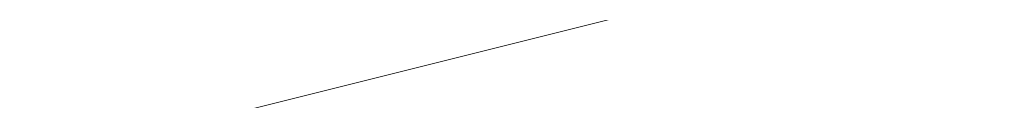
# Model space of a CAD drawing. Units: inches. Extents: x 2091 to 2899, y 967 to 2217.
# Tile 98 of 256: x 2251.243 to 2252.382, y 1099.986 to 1100.071. Entities that reach past the tile are written whole.
import ezdxf

# ---------------------------------------------------------------- set-up
doc = ezdxf.new("R2010")
doc.units = ezdxf.units.IN
doc.layers.add('A-ANNO-DIMS', color=2, linetype='Continuous', lineweight=18)
doc.layers.add('L-PLNT-TREE', color=94, linetype='Continuous', lineweight=13)
doc.layers.add('A-WALL-PATT', color=141, linetype='Continuous', lineweight=13, true_color=0xadddf7)
doc.styles.get("Standard").update_dxf_attribs({"font": 'arial.ttf'})
doc.dimstyles.new('ISO-25', dxfattribs={"dimtxt": 4, "dimasz": 4, "dimexe": 1.25, "dimexo": 0.625, "dimtad": 1, "dimdec": 0, "dimlunit": 3, "dimtxsty": 'Standard', "dimcen": 2.5, "dimadec": 0, "dimazin": 0, "dimtfac": 1, "dimtdec": 0, "dimtmove": 0, "dimatfit": 3, "dimfxl": 1, "dimarcsym": 0})

# ---------------------------------------------------------------- blocks, each defined once
blk = doc.blocks.new('*U29')
blk.add_line((-402.336, 12.192), (-451.104, 0))
blk = doc.blocks.new('*D71')
at = {"layer": 'A-ANNO-DIMS', "color": 0, "lineweight": -2, "transparency": 16777216}
for p, q in [((2212.1436, 1351.2941), (2212.1436, 969.4643)), ((2452.1436, 1351.2941), (2452.1436, 969.4643)), ((2216.1436, 970.7143), (2448.1436, 970.7143))]:
    blk.add_line(p, q, dxfattribs=at)
at = {"layer": 'A-ANNO-DIMS', "color": 0, "transparency": 16777216}
for points in [[(2216.1436, 971.381), (2216.1436, 970.0476), (2212.1436, 970.7143)], [(2448.1436, 971.381), (2448.1436, 970.0476), (2452.1436, 970.7143)]]:
    blk.add_solid(points, dxfattribs=at)
at = {"layer": 'Defpoints', "color": 0, "transparency": 16777216}
for p in [(2212.1436, 1351.9191), (2452.1436, 1351.9191), (2452.1436, 970.7143)]:
    blk.add_point(p, dxfattribs=at)
at = {"layer": 'A-ANNO-DIMS', "color": 0, "transparency": 16777216, "insert": (2332.1436, 973.3816), "char_height": 4, "attachment_point": 5}
blk.add_mtext('20\'-0"', dxfattribs=at)
blk = doc.blocks.new('*D75')
at = {"layer": 'A-ANNO-DIMS', "color": 0, "lineweight": -2, "transparency": 16777216}
for p, q in [((2212.1436, 1274.7941), (2212.1436, 969.4643)), ((2308.1436, 1274.7941), (2308.1436, 969.4643)), ((2216.1436, 970.7143), (2304.1436, 970.7143))]:
    blk.add_line(p, q, dxfattribs=at)
at = {"layer": 'A-ANNO-DIMS', "color": 0, "transparency": 16777216}
for points in [[(2216.1436, 971.381), (2216.1436, 970.0476), (2212.1436, 970.7143)], [(2304.1436, 971.381), (2304.1436, 970.0476), (2308.1436, 970.7143)]]:
    blk.add_solid(points, dxfattribs=at)
at = {"layer": 'Defpoints', "color": 0, "transparency": 16777216}
for p in [(2212.1436, 1275.4191), (2308.1436, 1275.4191), (2308.1436, 970.7143)]:
    blk.add_point(p, dxfattribs=at)
at = {"layer": 'A-ANNO-DIMS', "color": 0, "transparency": 16777216, "insert": (2260.1436, 973.3816), "char_height": 4, "attachment_point": 5}
blk.add_mtext('8\'-0"', dxfattribs=at)

msp = doc.modelspace()

# ---------------------------------------------------------------- hatches: boundary and pattern name
at = {"layer": 'A-WALL-PATT'}
h = msp.add_hatch(color=256, dxfattribs=at)
h.dxf.hatch_style = 1
h.paths.add_polyline_path([(2803.1436, 2050.9191), (2203.1436, 2050.9191), (2203.1436, 1090.9191), (2803.1436, 1090.9191)])
h.paths.add_polyline_path([(2635.7989, 1147.5405), (2674.5241, 1147.5405, 0.376086), (2678.5297, 1152.8802), (2678.5297, 1159.5565, 0.333335), (2674.5243, 1163.5618), (2674.5243, 1163.5619), (2674.5243, 1192.9344), (2635.806, 1192.9344), (2597.0876, 1192.9344), (2597.0876, 1163.5618, 0.333335), (2593.0823, 1159.5565), (2593.0823, 1152.8802, 0.376086), (2597.0879, 1147.5405)], flags=0)
h.paths.add_polyline_path([(2436.0104, 1278.2408, 0.000483), (2435.9526, 1278.215, -0.001328), (2435.9356, 1278.1117, -0.001711), (2436.1164, 1278.0408, 0.002185)], flags=0)
h.paths.add_polyline_path([(2794.1436, 1143.4191), (2794.1436, 1347.4191), (2543.3702, 1347.4191), (2543.3702, 1351.9191), (2794.1436, 1351.9191), (2794.1436, 1392.7136), (2793.9474, 1392.7136), (2793.9474, 1473.5369), (2794.1436, 1473.5369), (2794.1436, 1531.9191), (2650.1436, 1531.9191), (2650.1436, 1536.4191), (2794.1436, 1536.4191), (2794.1436, 1692.4191), (2609.3756, 1692.4191), (2609.3756, 1644.4191), (2604.8756, 1644.4191), (2604.8756, 1744.9191), (2609.3756, 1744.9191), (2609.3756, 1696.9191), (2794.1436, 1696.9191), (2794.1436, 1780.9191), (2609.6436, 1780.9191), (2493.8756, 1780.9191), (2493.8756, 1785.4191), (2609.6436, 1785.4191), (2794.1436, 1785.4191), (2794.1436, 1847.9388), (2793.9512, 1847.9388), (2793.9512, 1928.7622), (2794.1436, 1928.7622), (2794.1436, 1941.4191), (2614.1436, 1941.4191), (2614.1436, 1821.4191), (2609.6436, 1821.4191), (2609.6436, 1941.4191), (2392.1436, 1941.4191), (2392.1436, 1819.9191), (2387.6436, 1819.9191), (2387.6436, 1941.4191), (2212.1436, 1941.4191), (2212.1436, 1783.9191), (2392.1436, 1783.9191), (2392.1436, 1780.9191), (2212.1436, 1780.9191), (2212.1436, 1629.4191), (2387.6436, 1629.4191), (2387.6436, 1744.9191), (2392.1436, 1744.9191), (2392.1436, 1627.9191), (2317.1436, 1627.9191), (2317.1436, 1551.4191), (2317.1436, 1536.4191), (2459.3836, 1536.4191), (2459.3836, 1602.3965), (2463.8836, 1602.3965), (2463.8836, 1531.9191), (2456.6436, 1531.9191), (2456.6436, 1529.9191), (2452.1436, 1529.9191), (2452.1436, 1531.9191), (2312.6436, 1531.9191), (2312.6436, 1551.4191), (2306.1436, 1551.4191), (2306.1436, 1555.9191), (2308.1436, 1555.9191), (2308.1436, 1551.4191), (2312.6436, 1551.4191), (2312.6436, 1627.9191), (2212.1436, 1627.9191), (2212.1436, 1555.9191), (2270.1436, 1555.9191), (2270.1436, 1551.4191), (2212.1436, 1551.4191), (2212.1436, 1351.9191), (2272.1436, 1351.9191), (2272.1436, 1347.4191), (2212.1436, 1347.4191), (2212.1436, 1275.4191), (2308.1436, 1275.4191), (2308.1436, 1351.9191), (2452.1436, 1351.9191), (2452.1436, 1493.9191), (2456.6436, 1493.9191), (2456.6436, 1347.4191), (2312.6436, 1347.4191), (2312.6436, 1270.9191), (2212.1436, 1270.9191), (2212.1436, 1099.9191), (2281.2375, 1099.9191), (2282.871, 1110.9138), (2282.0083, 1116.9966), (2278.5577, 1121.4204), (2268.2056, 1128.0562), (2272.0876, 1128.0562), (2273.8129, 1131.927), (2279.4203, 1134.6919), (2285.0278, 1135.2449), (2287.6158, 1137.4568), (2288.0471, 1138.0098), (2289.3411, 1140.7747), (2291.0665, 1139.6687), (2292.3605, 1135.2449), (2295.3798, 1136.9038), (2296.2425, 1135.7979), (2297.1052, 1133.033), (2300.1246, 1138.0098), (2303.1439, 1138.0098), (2304.4379, 1135.7979), (2303.1439, 1133.586), (2306.5946, 1134.6919), (2307.8887, 1133.033), (2310.908, 1135.2449), (2313.9274, 1134.1389), (2315.6269, 1132.4271), (2308.32, 1117.5496), (2290.2038, 1109.8079), (2288.9098, 1103.1721), (2289.2723, 1099.9191), (2434.9182, 1099.9191), (2431.5932, 1124.7881), (2429.9302, 1169.5531), (2430.9272, 1240.5197), (2435.6589, 1238.1861), (2437.1352, 1196.5541), (2438.7982, 1143.9731), (2442.6782, 1111.9981), (2446.5582, 1099.9191), (2794.1436, 1099.9191), (2794.1436, 1138.9191), (2548.0324, 1138.9191), (2548.0324, 1143.4191), (2548.0324, 1148.8191), (2546.6685, 1148.0316), (2528.6857, 1179.1786, 0.256256), (2512.0324, 1148.8191), (2512.0324, 1143.4191), (2512.0324, 1138.9191), (2507.5324, 1138.9191), (2507.5324, 1143.4191), (2507.5324, 1148.8191, 0.256256), (2490.8792, 1179.1786), (2472.8964, 1148.0316), (2471.5324, 1148.8191), (2471.5324, 1143.4191), (2467.0324, 1143.4191), (2467.0324, 1269.9458, 0.039061), (2460.91, 1273.5801), (2467.0324, 1273.5801), (2467.0324, 1286.3254, 0.014511), (2465.2162, 1286.7619), (2467.0324, 1287.0526), (2467.0324, 1323.4191), (2471.5324, 1323.4191), (2471.5324, 1148.8191), (2489.5324, 1179.996), (2490.8964, 1179.2085), (2490.8792, 1179.1786, -0.256256), (2507.5324, 1148.8191), (2507.5324, 1143.4191), (2512.0324, 1143.4191), (2512.0324, 1148.8191, -0.256256), (2528.6857, 1179.1786), (2528.6685, 1179.2085), (2530.0324, 1179.996), (2548.0324, 1148.8191), (2548.0324, 1143.4191)], flags=16)
h.paths.add_polyline_path([(2607.7685, 1200.9451), (2607.7685, 1265.0306), (2597.0876, 1281.052), (2619.7846, 1281.052), (2627.7953, 1337.1269), (2635.7989, 1337.1269), (2643.8167, 1337.1269), (2651.8274, 1281.052), (2674.5243, 1281.052), (2663.8434, 1265.0306), (2663.8434, 1200.9451), (2635.806, 1200.9451)], flags=0)
edge = h.paths.add_edge_path(flags=0)
edge.add_ellipse((13303.8962, 1272.9987), major_axis=(-10595.313, 0), ratio=0.8423038701, start_angle=0.62823722, end_angle=0.6465541, ccw=False)
edge.add_ellipse((2711.7004, 1156.8527), major_axis=(2.2198, 0), ratio=0.842304, start_angle=111.5352, end_angle=180.6282, ccw=False)
edge.add_ellipse((13303.1563, 1272.9987), major_axis=(-10593.0263, 0), ratio=0.8423038695, start_angle=0.52827147, end_angle=0.6465541, ccw=False)
edge.add_line((2710.7646, 1175.3333), (2710.13, 1175.3333))
edge.add_ellipse((2710.13, 1176.5798), major_axis=(1.4798, 0), ratio=0.842304, start_angle=180, end_angle=270, ccw=False)
edge.add_line((2708.6501, 1176.5798), (2708.6501, 1200.7829))
edge.add_ellipse((2710.13, 1200.7829), major_axis=(1.4798, 0), ratio=0.842304, start_angle=90, end_angle=180, ccw=False)
edge.add_line((2710.13, 1202.0294), (2710.4651, 1202.0294))
edge.add_ellipse((13303.1563, 1272.9987), major_axis=(-10593.0263, 0), ratio=0.8423038695, start_angle=-0.09022909, end_angle=0.38386678, ccw=False)
edge.add_ellipse((2710.13, 1290.927), major_axis=(-1.4798, 0), ratio=0.842304, start_angle=0, end_angle=90, ccw=False)
edge.add_line((2708.6501, 1290.927), (2708.6501, 1315.1302))
edge.add_ellipse((2710.13, 1315.1302), major_axis=(-1.4798, 0), ratio=0.842304, start_angle=-90, end_angle=0, ccw=False)
edge.add_line((2710.13, 1316.3767), (2710.7063, 1316.3767))
edge.add_ellipse((3238.4017, 1296.2896), major_axis=(528.234, 0), ratio=0.84230387, start_angle=176.349572, end_angle=177.82005, ccw=False)
edge.add_ellipse((2775.063, 1071.4507), major_axis=(313.3078, 0), ratio=0.84230387, start_angle=102.125966, end_angle=103.780529, ccw=False)
edge.add_ellipse((2775.063, 1078.3057), major_axis=(-305.3029, 0), ratio=0.84230387, start_angle=-79.790461, end_angle=-77.555373, ccw=False)
edge.add_ellipse((2695.1418, 1541.9754), major_axis=(-250.9602, 0), ratio=0.84230387, start_angle=99.256566, end_angle=102.554933)
edge.add_line((2741.4103, 1334.2143), (2747.1325, 1337.3785))
edge.add_ellipse((2747.5386, 1336.8575), major_axis=(-0.7399, 0), ratio=0.842304, start_angle=270, end_angle=307.9331, ccw=False)
edge.add_ellipse((2747.5386, 1336.8575), major_axis=(-0.7399, 0), ratio=0.842304, start_angle=232.0669, end_angle=270, ccw=False)
edge.add_line((2747.9447, 1337.3785), (2753.6669, 1334.2143))
edge.add_ellipse((2799.9355, 1541.9754), major_axis=(250.9602, 0), ratio=0.84230387, start_angle=257.445067, end_angle=260.743434)
edge.add_ellipse((2720.0142, 1078.3057), major_axis=(305.3029, 0), ratio=0.84230387, start_angle=77.555373, end_angle=79.790461, ccw=False)
edge.add_ellipse((2720.0142, 1071.4507), major_axis=(-313.3078, 0), ratio=0.84230387, start_angle=256.219471, end_angle=257.874034, ccw=False)
edge.add_ellipse((2256.6755, 1296.2896), major_axis=(-528.234, 0), ratio=0.84230387, start_angle=182.17995, end_angle=183.650428, ccw=False)
edge.add_line((2784.3709, 1316.3767), (2784.9472, 1316.3767))
edge.add_ellipse((2784.9472, 1315.1302), major_axis=(1.4798, 0), ratio=0.842304, start_angle=0, end_angle=90, ccw=False)
edge.add_line((2786.4271, 1315.1302), (2786.4271, 1290.927))
edge.add_ellipse((2784.9472, 1290.927), major_axis=(1.4798, 0), ratio=0.842304, start_angle=270, end_angle=360, ccw=False)
edge.add_ellipse((-7808.0791, 1272.9987), major_axis=(10593.0263, 0), ratio=0.8423038695, start_angle=-0.38386678, end_angle=0.09022909, ccw=False)
edge.add_line((2784.6122, 1202.0294), (2784.9472, 1202.0294))
edge.add_ellipse((2784.9472, 1200.7829), major_axis=(1.4798, 0), ratio=0.842304, start_angle=0, end_angle=90, ccw=False)
edge.add_line((2786.4271, 1200.7829), (2786.4271, 1176.5798))
edge.add_ellipse((2784.9472, 1176.5798), major_axis=(-1.4798, 0), ratio=0.842304, start_angle=90, end_angle=180, ccw=False)
edge.add_line((2784.9472, 1175.3333), (2784.3126, 1175.3333))
edge.add_ellipse((-7808.0791, 1272.9987), major_axis=(10593.0263, 0), ratio=0.8423038695, start_angle=-0.6186432, end_angle=-0.52827147, ccw=False)
edge.add_ellipse((2783.3768, 1156.8527), major_axis=(-2.2198, 0), ratio=0.842304, start_angle=179.3718, end_angle=248.4648, ccw=False)
edge.add_ellipse((-7808.819, 1272.9987), major_axis=(-10595.313, 0), ratio=0.8423038658, start_angle=179.35344592, end_angle=179.3717628, ccw=False)
edge.add_ellipse((2780.2973, 1153.5008), major_axis=(-5.2464, 0), ratio=0.842304, start_angle=90, end_angle=179.3534, ccw=False)
edge.add_line((2780.2973, 1149.0817), (2714.7799, 1149.0817))
edge.add_ellipse((2714.7799, 1153.5008), major_axis=(5.2464, 0), ratio=0.842304, start_angle=180.6466, end_angle=270, ccw=False)
edge = h.paths.add_edge_path(flags=0)
edge.add_line((2718.1874, 1151.0078), (2718.1874, 1170.4724))
edge.add_ellipse((2721.1471, 1170.4724), major_axis=(-2.9597, 0), ratio=0.842304, start_angle=-90, end_angle=0, ccw=False)
edge.add_line((2721.1471, 1172.9653), (2773.9302, 1172.9653))
edge.add_ellipse((2773.9302, 1170.4724), major_axis=(-2.9597, 0), ratio=0.842304, start_angle=180, end_angle=270, ccw=False)
edge.add_line((2776.8899, 1170.4724), (2776.8899, 1151.0078))
edge.add_line((2776.8899, 1151.0078), (2718.1874, 1151.0078))
edge = h.paths.add_edge_path(flags=0)
edge.add_line((2718.1874, 1180.2342), (2718.1874, 1199.0578))
edge.add_ellipse((2747.5386, 1320.3986), major_axis=(147.0179, 0), ratio=0.84230387, start_angle=256.401865, end_angle=283.598135)
edge.add_line((2776.8899, 1199.0578), (2776.8899, 1180.2342))
edge.add_ellipse((2747.5386, 1301.575), major_axis=(147.0179, 0), ratio=0.84230387, start_angle=256.401865, end_angle=283.598135, ccw=False)
edge = h.paths.add_edge_path(flags=0)
edge.add_ellipse((13303.1563, 1272.9987), major_axis=(-10591.5465, 0), ratio=0.8423038696, start_angle=0.05559431, end_angle=0.37776419, ccw=False)
edge.add_line((2711.6169, 1262.7217), (2715.6674, 1249.4954))
edge.add_ellipse((6413.892, 1241.6919), major_axis=(-3698.2362, 0), ratio=0.84230387, start_angle=-0.1208974, end_angle=0.3640763)
edge.add_line((2715.761, 1218.1925), (2711.9343, 1203.1674))
edge = h.paths.add_edge_path(flags=0)
edge.add_line((2718.1874, 1251.0746), (2716.0025, 1267.4504))
edge.add_ellipse((2742.1512, 1202.1895), major_axis=(81.7726, 0), ratio=0.8423039, start_angle=94.277421, end_angle=111.834954, ccw=False)
edge.add_line((2737.0097, 1270.9306), (2758.0675, 1270.9306))
edge.add_ellipse((2752.9261, 1202.1895), major_axis=(81.7726, 0), ratio=0.8423039, start_angle=68.165046, end_angle=85.722579, ccw=False)
edge.add_line((2779.0747, 1267.4504), (2776.8899, 1251.0746))
edge.add_ellipse((2750.3381, 1187.8854), major_axis=(79.5797, 0), ratio=0.8423039, start_angle=67.208085, end_angle=85.12993)
edge.add_line((2756.0347, 1254.7437), (2739.0426, 1254.7437))
edge.add_ellipse((2744.7392, 1187.8854), major_axis=(79.5797, 0), ratio=0.8423039, start_angle=94.87007, end_angle=112.791915)
edge = h.paths.add_edge_path(flags=0)
edge.add_line((2783.1429, 1203.1674), (2779.3162, 1218.1925))
edge.add_ellipse((-918.8147, 1241.6919), major_axis=(3698.2362, 0), ratio=0.84230387, start_angle=-0.3640763, end_angle=0.1208974)
edge.add_line((2779.4098, 1249.4954), (2783.4604, 1262.7217))
edge.add_ellipse((-7808.0791, 1272.9987), major_axis=(-10591.5465, 0), ratio=0.8423038695, start_angle=179.62223581, end_angle=179.94440569, ccw=False)
edge = h.paths.add_edge_path(flags=0)
edge.add_ellipse((2734.2009, 1286.6904), major_axis=(-0.3566, 6.3401), ratio=0.603834, start_angle=89.00201, end_angle=253.65741, ccw=False)
edge.add_line((2730.369, 1286.5418), (2730.369, 1301.352))
edge.add_line((2730.369, 1301.352), (2735.9133, 1305.2148))
edge.add_ellipse((2736.3849, 1304.7346), major_axis=(0.7399, 0), ratio=0.842304, start_angle=90, end_angle=134.4802, ccw=False)
edge.add_line((2736.3849, 1305.3578), (2738.0328, 1305.3578))
edge.add_line((2738.0328, 1305.3578), (2738.0328, 1307.7079))
edge.add_ellipse((2794.2016, 1307.7079), major_axis=(56.1689, 0), ratio=0.8423039, start_angle=150.56143, end_angle=180, ccw=False)
edge.add_ellipse((2700.8756, 1307.7079), major_axis=(-56.1689, 0), ratio=0.8423039, start_angle=180, end_angle=209.43857, ccw=False)
edge.add_line((2757.0444, 1307.7079), (2757.0444, 1305.3578))
edge.add_line((2757.0444, 1305.3578), (2758.6923, 1305.3578))
edge.add_ellipse((2758.6923, 1304.7346), major_axis=(-0.7399, 0), ratio=0.842304, start_angle=225.5198, end_angle=270, ccw=False)
edge.add_line((2759.1639, 1305.2148), (2764.7082, 1301.352))
edge.add_line((2764.7082, 1301.352), (2764.7082, 1286.5418))
edge.add_ellipse((2760.8763, 1286.6904), major_axis=(0.3566, 6.3401), ratio=0.603834, start_angle=106.34259, end_angle=270.99799, ccw=False)
edge.add_line((2757.0444, 1285.7971), (2757.0444, 1307.7079))
edge.add_ellipse((2700.8756, 1307.7079), major_axis=(-56.1689, 0), ratio=0.8423039, start_angle=180, end_angle=209.43857)
edge.add_ellipse((2794.2016, 1307.7079), major_axis=(56.1689, 0), ratio=0.8423039, start_angle=150.56143, end_angle=180)
edge.add_line((2738.0328, 1307.7079), (2738.0328, 1285.7971))
h.paths.add_polyline_path([(2417.8123, 1104.4497), (2413.4923, 1102.5297), (2410.6123, 1103.9697), (2409.1723, 1106.3697), (2407.2523, 1107.3297), (2406.2923, 1109.7297), (2405.3323, 1114.0497), (2405.3323, 1117.8897), (2406.2923, 1120.1297), (2407.2523, 1119.8097), (2408.8483, 1118.3277), (2410.1739, 1119.4242), (2410.2113, 1120.4057), (2411.0407, 1121.4191), (2410.6993, 1119.8587), (2410.1739, 1119.4242), (2410.0885, 1117.1761), (2411.1328, 1116.2063), (2413.9723, 1119.3297), (2416.8523, 1120.7697), (2416.8697, 1120.7988), (2417.0351, 1119.4051), (2417.8962, 1118.1434), (2418.2923, 1118.3697), (2419.5444, 1120.0393), (2419.3609, 1118.3875), (2419.0321, 1119.3562), (2418.3989, 1118.5119), (2419.2523, 1114.5297), (2418.7941, 1107.1988)], flags=0)
h.paths.add_polyline_path([(2508.8702, 1347.4191), (2508.3702, 1347.4191), (2508.3702, 1351.9191), (2508.8702, 1351.9191)], flags=0)
h.paths.add_polyline_path([(2473.3702, 1347.4191), (2472.3702, 1347.4191), (2467.8702, 1347.4191), (2467.8702, 1455.4191), (2472.3702, 1455.4191), (2472.3702, 1352.4191), (2473.3702, 1352.4191)], flags=0)
h.paths.add_polyline_path([(2352.1062, 1217.4462), (2349.2262, 1218.8862), (2347.7862, 1221.2862), (2345.8662, 1222.2462), (2344.9062, 1224.6462), (2343.9462, 1228.9662), (2343.9462, 1232.8062), (2344.9062, 1235.0462), (2345.8662, 1234.7262), (2347.4623, 1233.2442), (2348.7879, 1234.3407), (2348.8252, 1235.3222), (2349.6547, 1236.3355), (2349.3132, 1234.7752), (2348.7879, 1234.3407), (2348.7024, 1232.0926), (2349.7468, 1231.1228), (2352.5862, 1234.2462), (2355.4662, 1235.6862), (2355.4837, 1235.7153), (2355.649, 1234.3216), (2356.5102, 1233.0599), (2356.9062, 1233.2862), (2358.1584, 1234.9558), (2357.9749, 1233.304), (2357.6461, 1234.2726), (2357.0129, 1233.4284), (2357.8662, 1229.4462), (2357.4081, 1222.1153), (2356.4262, 1219.3662)], flags=0)
h.paths.add_polyline_path([(2348.2968, 1112.2244), (2347.0138, 1112.3104), (2345.5298, 1114.1274), (2345.7318, 1115.8584), (2346.8118, 1116.9824), (2346.8118, 1114.6464), (2345.8668, 1114.2144), (2346.8798, 1114.3004)], flags=0)
h.paths.add_polyline_path([(2347.0138, 1110.9264), (2346.2718, 1110.4934), (2346.6098, 1111.1864)], flags=0)
h.paths.add_polyline_path([(2345.8668, 1118.1944), (2345.5298, 1117.3294), (2343.7078, 1118.0214), (2344.3828, 1118.6264)], flags=0)
h.paths.add_polyline_path([(2346.6768, 1109.2824), (2346.0698, 1108.0714), (2345.8668, 1110.0614)], flags=0)
h.paths.add_polyline_path([(2345.0568, 1119.7514), (2343.6398, 1119.7514), (2343.9778, 1121.1354)], flags=0)
h.paths.add_polyline_path([(2345.2598, 1116.5504), (2345.1248, 1115.8584), (2344.9218, 1115.6854), (2344.7198, 1116.3774)], flags=0)
h.paths.add_polyline_path([(2345.6648, 1112.3104), (2345.4618, 1111.5324), (2344.0448, 1111.9644), (2344.6518, 1112.5704)], flags=0)
h.paths.add_polyline_path([(2345.1918, 1113.3494), (2344.4498, 1113.8684), (2344.7198, 1114.3874)], flags=0)
h.paths.add_polyline_path([(2344.6518, 1116.8094), (2344.1798, 1115.6854), (2344.6518, 1115.3394), (2343.9098, 1114.9064), (2343.0328, 1115.9444), (2343.6398, 1116.4634)], flags=0)
h.paths.add_polyline_path([(2345.8668, 1106.6864), (2344.9898, 1105.5624), (2344.5168, 1106.6004)], flags=0)
h.paths.add_polyline_path([(2344.8548, 1110.0614), (2344.5168, 1109.2824), (2344.1128, 1109.7154)], flags=0)
h.paths.add_polyline_path([(2344.0448, 1113.5224), (2343.4378, 1113.0894), (2342.7628, 1113.9544)], flags=0)
h.paths.add_polyline_path([(2344.3148, 1111.0124), (2342.9648, 1110.3204), (2342.9648, 1111.0994)], flags=0)
h.paths.add_polyline_path([(2345.1248, 1104.6974), (2344.5848, 1103.7454), (2344.4498, 1104.2644)], flags=0)
h.paths.add_polyline_path([(2342.8298, 1121.2224), (2341.7498, 1120.5304), (2340.5358, 1121.0494), (2340.1308, 1121.8284), (2340.6708, 1122.9524), (2341.1428, 1121.8284), (2341.6148, 1122.0014)], flags=0)
h.paths.add_polyline_path([(2342.9648, 1119.7514), (2343.0328, 1118.4534), (2342.0878, 1118.0214), (2342.0198, 1119.4914)], flags=0)
h.paths.add_polyline_path([(2342.6948, 1116.8964), (2341.9528, 1116.6364), (2342.0198, 1117.3294)], flags=0)
h.paths.add_polyline_path([(2343.0328, 1112.2244), (2342.0198, 1111.7914), (2341.5478, 1112.2244), (2342.3578, 1113.3494)], flags=0)
h.paths.add_polyline_path([(2343.7748, 1104.4374), (2342.6278, 1102.8804), (2342.6948, 1104.6104), (2343.4378, 1105.1294)], flags=0)
h.paths.add_polyline_path([(2342.0198, 1115.0794), (2340.8058, 1115.5124), (2340.9408, 1116.3774)], flags=0)
h.paths.add_polyline_path([(2341.4808, 1120.0974), (2341.4808, 1119.4054), (2341.0758, 1119.5784), (2341.1428, 1120.0974)], flags=0)
h.paths.add_polyline_path([(2341.8178, 1114.4734), (2340.9408, 1113.0894), (2340.8058, 1114.5604)], flags=0)
h.paths.add_polyline_path([(2341.1428, 1118.5404), (2340.9408, 1116.9824), (2339.0508, 1117.6754), (2339.0508, 1118.6264)], flags=0)
h.paths.add_polyline_path([(2342.6948, 1101.6684), (2341.9528, 1101.8414), (2342.5598, 1102.3614)], flags=0)
h.paths.add_polyline_path([(2340.3328, 1119.6654), (2338.4438, 1119.5784), (2337.9038, 1120.3574), (2339.6578, 1120.6164)], flags=0)
h.paths.add_polyline_path([(2340.3328, 1115.3394), (2340.0628, 1113.6954), (2339.3878, 1115.3394)], flags=0)
h.paths.add_polyline_path([(2341.8178, 1103.8314), (2341.5478, 1102.8804), (2341.1428, 1103.6584)], flags=0)
h.paths.add_polyline_path([(2339.0508, 1122.8664), (2337.2958, 1121.8284), (2337.0938, 1123.1254), (2337.7688, 1123.8184)], flags=0)
h.paths.add_polyline_path([(2339.1178, 1121.7414), (2338.8478, 1121.2224), (2338.1738, 1121.0494), (2338.3758, 1121.5684)], flags=0)
h.paths.add_polyline_path([(2339.1858, 1119.3194), (2338.6458, 1118.7134), (2338.2408, 1118.1074), (2338.2408, 1118.8864)], flags=0)
h.paths.add_polyline_path([(2341.1428, 1101.9284), (2340.6028, 1101.2364), (2340.0628, 1101.8414), (2340.6028, 1102.3614)], flags=0)
h.paths.add_polyline_path([(2337.6338, 1117.7614), (2336.6208, 1118.2804), (2337.2958, 1118.9724)], flags=0)
h.paths.add_polyline_path([(2336.8238, 1119.5784), (2334.7988, 1118.9724), (2335.2038, 1120.3574), (2336.5538, 1120.8764)], flags=0)
h.paths.add_polyline_path([(2339.1178, 1100.4574), (2337.3638, 1100.5434), (2336.7558, 1101.2364)], flags=0)
h.paths.add_polyline_path([(2336.3508, 1122.4334), (2336.0138, 1121.9144), (2334.9338, 1122.4334), (2334.5288, 1123.4714), (2335.7438, 1122.7794)], flags=0)
h.paths.add_polyline_path([(2334.7318, 1120.8764), (2334.2588, 1120.3574), (2334.0568, 1120.7894), (2334.5968, 1121.3084)], flags=0)
h.paths.add_polyline_path([(2334.4618, 1122.1744), (2332.5718, 1121.3084), (2331.3568, 1122.1744), (2332.0998, 1122.8664)], flags=0)
h.paths.add_polyline_path([(2334.2588, 1118.5404), (2333.3818, 1118.4534), (2333.6518, 1119.3194)], flags=0)
h.paths.add_polyline_path([(2335.5418, 1102.2744), (2334.1918, 1102.6204), (2335.2718, 1103.3124)], flags=0)
h.paths.add_polyline_path([(2332.7068, 1119.6654), (2331.6948, 1120.4434), (2332.5048, 1120.7894)], flags=0)
h.paths.add_polyline_path([(2334.7318, 1101.1494), (2333.5168, 1101.5824), (2333.9888, 1101.7554)], flags=0)
h.paths.add_polyline_path([(2332.6398, 1116.6364), (2331.0868, 1116.2904), (2331.9648, 1118.1944)], flags=0)
h.paths.add_polyline_path([(2330.7498, 1121.5684), (2330.2768, 1120.2704), (2328.5228, 1119.3194), (2328.9948, 1121.0494)], flags=0)
h.paths.add_polyline_path([(2330.7498, 1118.6264), (2330.0078, 1117.5024), (2329.8728, 1118.0214)], flags=0)
h.paths.add_polyline_path([(2332.0998, 1102.3614), (2330.5468, 1102.0144), (2331.6948, 1102.9664)], flags=0)
h.paths.add_polyline_path([(2329.5348, 1113.6084), (2329.0628, 1112.3104), (2328.5898, 1113.3494)], flags=0)
h.paths.add_polyline_path([(2328.3878, 1117.8484), (2327.5098, 1116.5504), (2327.1728, 1117.7614)], flags=0)
h.paths.add_polyline_path([(2329.7378, 1106.5134), (2329.5348, 1105.3024), (2328.2528, 1106.0814)], flags=0)
h.paths.add_polyline_path([(2328.6578, 1114.3874), (2328.0498, 1114.1274), (2328.3198, 1114.9064)], flags=0)
h.paths.add_polyline_path([(2328.3198, 1112.2244), (2327.1058, 1112.1374), (2326.7008, 1112.6564)], flags=0)
h.paths.add_polyline_path([(2326.9028, 1115.2524), (2326.7008, 1114.1274), (2325.2158, 1113.6084), (2326.0928, 1115.3394)], flags=0)
h.paths.add_polyline_path([(2326.6328, 1108.3304), (2326.0928, 1107.3794), (2325.8908, 1108.5034), (2326.4978, 1109.1094)], flags=0)
h.paths.add_polyline_path([(2615.1436, 1531.9191), (2609.6436, 1531.9191), (2609.6436, 1620.4191), (2614.1436, 1620.4191), (2614.1436, 1536.4191), (2615.1436, 1536.4191)], flags=0)
h.paths.add_polyline_path([(2545.1436, 1563.4191), (2464.1436, 1563.4191), (2464.1436, 1632.4191), (2509.1436, 1632.4191), (2509.1436, 1627.9191), (2509.1436, 1603.9191), (2468.6436, 1603.9191), (2468.6436, 1567.9191), (2540.6436, 1567.9191), (2540.6436, 1591.9191), (2545.1436, 1591.9191)], flags=0)
h.paths.add_polyline_path([(2388.969, 1549.9857), (2357.4342, 1549.9857), (2357.4342, 1623.3608), (2399.3628, 1623.3608), (2435.6895, 1623.3608), (2435.5925, 1602.5593), (2435.5925, 1602.3965), (2388.969, 1602.3965)], flags=0)
h.paths.add_polyline_path([(2388.8806, 1555.8092), (2374.9044, 1555.8092), (2374.9044, 1600.5716), (2374.9044, 1615.4576), (2406.3509, 1615.4576), (2406.3509, 1618.9394), (2412.1743, 1615.4576), (2406.3509, 1611.9759), (2406.3509, 1615.4576), (2388.8806, 1615.4576)], flags=0)
h.paths.add_polyline_path([(2568.8756, 1644.4191), (2453.3756, 1644.4191), (2453.3756, 1785.4191), (2457.8756, 1785.4191), (2457.8756, 1648.9191), (2568.8756, 1648.9191)], flags=0)
h.paths.add_polyline_path([(2212.1436, 1945.9191), (2212.1436, 2041.9191), (2794.1436, 2041.9191), (2794.1436, 1945.9191)], flags=16)
h.paths.add_polyline_path([(2271.0827, 1964.3172), (2776.853, 1964.3172), (2776.853, 2037.1696), (2271.0827, 2037.1696)], flags=8)
h.paths.add_polyline_path([(2380.6493, 1536.8241), (2461.0408, 1536.8241), (2461.0408, 1554.6526), (2380.6493, 1554.6526)], flags=8)
h.paths.add_polyline_path([(2240.7557, 1609.7255), (2309.1858, 1609.7255), (2309.1858, 1617.6982), (2240.7557, 1617.6982)], flags=8)
h.paths.add_polyline_path([(2212.6773, 1313.5041), (2282.5915, 1313.5041), (2282.5915, 1322.7452), (2212.6773, 1322.7452)], flags=8)
h.paths.add_polyline_path([(2457.112, 1114.7786), (2558.4816, 1114.7786), (2558.4816, 1142.2197), (2457.112, 1142.2197)], flags=8)
h.paths.add_polyline_path([(2473.4423, 1273.0101), (2604.6412, 1273.0101), (2604.6412, 1318.3469), (2473.4423, 1318.3469)], flags=8)
h.paths.add_polyline_path([(2638.8763, 1626.9774), (2684.2504, 1627.9767), (2684.0385, 1637.5975), (2638.6644, 1636.5982)], flags=8)
h.paths.add_polyline_path([(2537.5906, 1453.7934), (2628.3895, 1453.7934), (2628.3895, 1475.3448), (2537.5906, 1475.3448)], flags=8)
h.paths.add_polyline_path([(2504.1376, 1714.6324), (2554.6472, 1714.6324), (2554.6472, 1730.2377), (2504.1376, 1730.2377)], flags=8)
h.paths.add_polyline_path([(2487.5012, 1575.6519), (2535.0971, 1575.6519), (2535.0971, 1598.3776), (2487.5012, 1598.3776)], flags=8)
h.paths.add_polyline_path([(2709.0994, 1735.7103), (2740.0166, 1735.7103), (2740.0166, 1749.9376), (2709.0994, 1749.9376)], flags=8)
h.paths.add_polyline_path([(2442.4384, 1792.1717), (2564.7288, 1792.1717), (2564.7288, 1842.0002), (2442.4384, 1842.0002)], flags=8)
h.paths.add_polyline_path([(2655.8158, 1809.6441), (2789.5201, 1806.6938), (2790.085, 1832.2916), (2656.3806, 1835.2419)], flags=8)
h.paths.add_polyline_path([(2234.8427, 1797.7201), (2368.5929, 1794.7689), (2369.1607, 1820.5041), (2235.4106, 1823.4554)], flags=8)
h.paths.add_polyline_path([(2245.1385, 1644.0063), (2398.4277, 1640.6239), (2398.9948, 1666.3248), (2245.7056, 1669.7073)], flags=8)
h.paths.add_polyline_path([(2306.1428, 1431.1685), (2413.7683, 1428.7937), (2414.3331, 1454.3915), (2306.7077, 1456.7664)], flags=8)
h.paths.add_polyline_path([(2306.8346, 1458.2331), (2393.3805, 1456.3234), (2393.9328, 1481.3544), (2307.3869, 1483.2641)], flags=8)

# ---------------------------------------------------------------- block references
at = {"layer": 'L-PLNT-TREE', "xscale": 0.0393700787401575, "yscale": 0.0393700787401575, "zscale": 0.0393700787401575}
msp.add_blockref('*U29', (2269.041, 1099.9191), dxfattribs=at)

# ---------------------------------------------------------------- dimensions: what is measured, and where the dimension line sits
at = {"layer": 'A-ANNO-DIMS'}
for base, p1, p2, picture, middle in [((2452.1436, 970.7143), (2212.1436, 1351.9191), (2452.1436, 1351.9191), '*D71', (2332.1436, 973.3816)), ((2308.1436, 970.7143), (2212.1436, 1275.4191), (2308.1436, 1275.4191), '*D75', (2260.1436, 973.3816))]:
    dim = msp.add_linear_dim(base=base, p1=p1, p2=p2, dimstyle='ISO-25', override={"dimdec": 1, "dimlfac": 1, "dimrnd": 0, "dimzin": 1, "dimdsep": 46, "dimlunit": 4, "dimfrac": 2}, dxfattribs=at)
    dim.commit()
    dim.dimension.update_dxf_attribs({"geometry": picture, "text_midpoint": middle})

doc.saveas('drawing.dxf')
